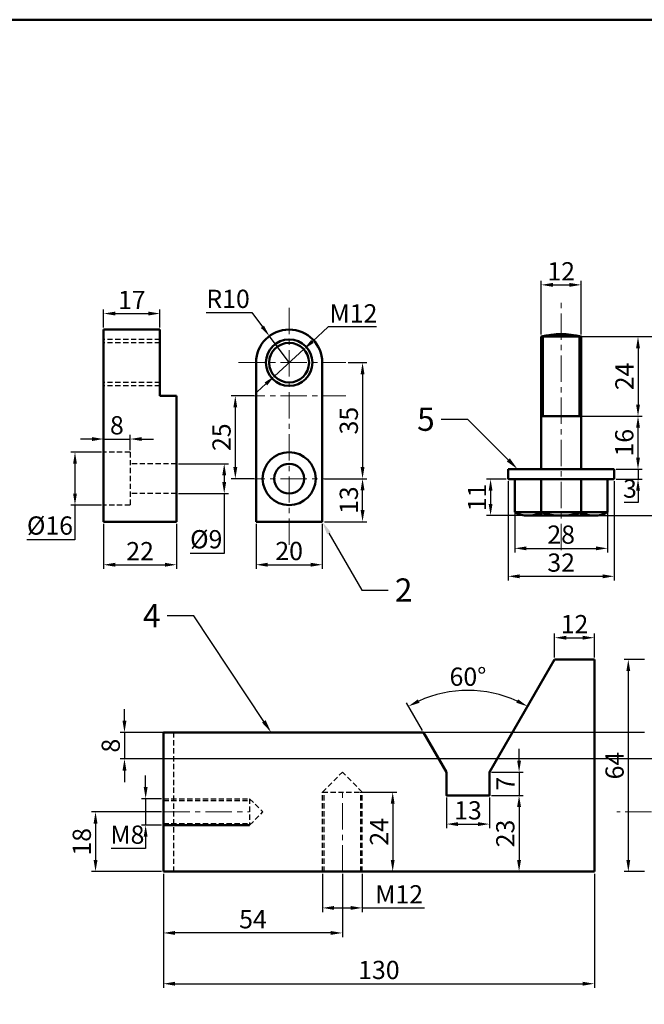
# Model space of a CAD drawing. Units: millimetres. Extents: x 10 to 613, y -226 to 271.
# Tile 3 of 4: x 251 to 439, y -26 to 271. Entities that reach past the tile are written whole.
import ezdxf
from ezdxf import colors
from ezdxf.entities.mleader import LeaderData, LeaderLine
from ezdxf.math import Vec2, Vec3

# ---------------------------------------------------------------- set-up
doc = ezdxf.new("R2010")
doc.units = ezdxf.units.MM
doc.header["$LTSCALE"] = 0.5
doc.linetypes.add('CENTER', pattern=[50.8, 31.75, -6.35, 6.35, -6.35])
doc.linetypes.add('HIDDEN', pattern=[9.525, 6.35, -3.175])
for name, color, linetype, lineweight in [('M-CNTR', 1, 'CENTER', 18), ('M-DIMS', 2, 'Continuous', 25), ('M-HIDN', 6, 'HIDDEN', 25), ('M-OUTL', 7, 'Continuous', 50), ('M-TTLB', 7, 'Continuous', 50)]:
    doc.layers.add(name, color=color, linetype=linetype, lineweight=lineweight)
doc.styles.get("Standard").update_dxf_attribs({"font": 'arial.ttf'})
doc.dimstyles.new('ISO-25', dxfattribs={"dimtxt": 5.5, "dimasz": 3.5, "dimexe": 1.25, "dimexo": 0.625, "dimtad": 1, "dimtoh": 1, "dimtxsty": 'Standard', "dimcen": 2.5, "dimadec": 0, "dimazin": 0, "dimtfac": 1, "dimtmove": 0, "dimatfit": 3, "dimfxl": 1, "dimarcsym": 0})

# ---------------------------------------------------------------- blocks, each defined once
blk = doc.blocks.new('*D5')
at = {"layer": 'Defpoints', "color": 0, "ltscale": 0.5, "transparency": 16777216}
for p in [(276.04, 140.19), (267.41, 124.19), (276.04, 124.19)]:
    blk.add_point(p, dxfattribs=at)
at = {"layer": 'M-DIMS', "color": 0, "lineweight": -2, "ltscale": 0.5, "transparency": 16777216}
for p, q in [((275.41, 140.19), (266.16, 140.19)), ((267.41, 136.69), (267.41, 127.69)), ((275.41, 124.19), (266.16, 124.19)), ((267.41, 124.19), (267.41, 113.75)), ((267.41, 113.75), (252.92, 113.75))]:
    blk.add_line(p, q, dxfattribs=at)
at = {"layer": 'M-DIMS', "color": 0, "ltscale": 0.5, "transparency": 16777216}
for points in [[(266.83, 136.69), (267.99, 136.69), (267.41, 140.19)], [(266.83, 127.69), (267.99, 127.69), (267.41, 124.19)]]:
    blk.add_solid(points, dxfattribs=at)
at = {"layer": 'M-DIMS', "color": 0, "ltscale": 0.5, "transparency": 16777216, "insert": (259.85, 117.34), "char_height": 5.5, "attachment_point": 5}
blk.add_mtext('%%C16', dxfattribs=at)
blk = doc.blocks.new('*D6')
at = {"layer": 'Defpoints', "color": 0, "ltscale": 0.5, "transparency": 16777216}
for p in [(284.04, 144.15), (276.04, 140.19), (284.04, 140.19)]:
    blk.add_point(p, dxfattribs=at)
at = {"layer": 'M-DIMS', "color": 0, "lineweight": -2, "ltscale": 0.5, "transparency": 16777216}
for p, q in [((272.54, 144.15), (269.04, 144.15)), ((276.04, 140.81), (276.04, 145.4)), ((276.04, 144.15), (284.04, 144.15)), ((284.04, 140.81), (284.04, 145.4)), ((287.54, 144.15), (291.04, 144.15))]:
    blk.add_line(p, q, dxfattribs=at)
at = {"layer": 'M-DIMS', "color": 0, "ltscale": 0.5, "transparency": 16777216}
for points in [[(272.54, 144.73), (272.54, 143.56), (276.04, 144.15)], [(287.54, 144.73), (287.54, 143.56), (284.04, 144.15)]]:
    blk.add_solid(points, dxfattribs=at)
at = {"layer": 'M-DIMS', "color": 0, "ltscale": 0.5, "transparency": 16777216, "insert": (280.04, 147.58), "char_height": 5.5, "attachment_point": 5}
blk.add_mtext('8', dxfattribs=at)
blk = doc.blocks.new('*D7')
at = {"layer": 'Defpoints', "color": 0, "ltscale": 0.5, "transparency": 16777216}
for p in [(293.04, 182), (276.04, 177.19), (293.04, 177.19)]:
    blk.add_point(p, dxfattribs=at)
at = {"layer": 'M-DIMS', "color": 0, "lineweight": -2, "ltscale": 0.5, "transparency": 16777216}
for p, q in [((276.04, 177.81), (276.04, 183.25)), ((279.54, 182), (289.54, 182)), ((293.04, 177.81), (293.04, 183.25))]:
    blk.add_line(p, q, dxfattribs=at)
at = {"layer": 'M-DIMS', "color": 0, "ltscale": 0.5, "transparency": 16777216}
for points in [[(279.54, 182.58), (279.54, 181.42), (276.04, 182)], [(289.54, 182.58), (289.54, 181.42), (293.04, 182)]]:
    blk.add_solid(points, dxfattribs=at)
at = {"layer": 'M-DIMS', "color": 0, "ltscale": 0.5, "transparency": 16777216, "insert": (284.54, 185.39), "char_height": 5.5, "attachment_point": 5}
blk.add_mtext('17', dxfattribs=at)
blk = doc.blocks.new('*D8')
at = {"layer": 'Defpoints', "color": 0, "ltscale": 0.5, "transparency": 16777216}
for p in [(298.04, 136.69), (298.04, 127.69), (312.42, 127.69)]:
    blk.add_point(p, dxfattribs=at)
at = {"layer": 'M-DIMS', "color": 0, "lineweight": -2, "ltscale": 0.5, "transparency": 16777216}
for p, q in [((298.66, 136.69), (313.67, 136.69)), ((312.42, 133.19), (312.42, 131.19)), ((298.66, 127.69), (313.67, 127.69)), ((312.42, 127.69), (312.42, 109.62)), ((312.42, 109.62), (302.2, 109.62))]:
    blk.add_line(p, q, dxfattribs=at)
at = {"layer": 'M-DIMS', "color": 0, "ltscale": 0.5, "transparency": 16777216}
for points in [[(311.84, 133.19), (313.01, 133.19), (312.42, 136.69)], [(311.84, 131.19), (313.01, 131.19), (312.42, 127.69)]]:
    blk.add_solid(points, dxfattribs=at)
at = {"layer": 'M-DIMS', "color": 0, "ltscale": 0.5, "transparency": 16777216, "insert": (307, 113.21), "char_height": 5.5, "attachment_point": 5}
blk.add_mtext('%%C9', dxfattribs=at)
blk = doc.blocks.new('*D9')
at = {"layer": 'Defpoints', "color": 0, "ltscale": 0.5, "transparency": 16777216}
for p in [(276.04, 119.19), (298.04, 119.19), (298.04, 106.22)]:
    blk.add_point(p, dxfattribs=at)
at = {"layer": 'M-DIMS', "color": 0, "lineweight": -2, "ltscale": 0.5, "transparency": 16777216}
for p, q in [((276.04, 118.56), (276.04, 104.97)), ((298.04, 118.56), (298.04, 104.97)), ((279.54, 106.22), (294.54, 106.22))]:
    blk.add_line(p, q, dxfattribs=at)
at = {"layer": 'M-DIMS', "color": 0, "ltscale": 0.5, "transparency": 16777216}
for points in [[(279.54, 106.81), (279.54, 105.64), (276.04, 106.22)], [(294.54, 106.81), (294.54, 105.64), (298.04, 106.22)]]:
    blk.add_solid(points, dxfattribs=at)
at = {"layer": 'M-DIMS', "color": 0, "ltscale": 0.5, "transparency": 16777216, "insert": (287.04, 109.61), "char_height": 5.5, "attachment_point": 5}
blk.add_mtext('22', dxfattribs=at)
blk = doc.blocks.new('*D10')
at = {"layer": 'Defpoints', "color": 0, "ltscale": 0.5, "transparency": 16777216}
for p in [(349.16, 167.19), (349.16, 132.19), (354.15, 132.19)]:
    blk.add_point(p, dxfattribs=at)
at = {"layer": 'M-DIMS', "color": 0, "lineweight": -2, "ltscale": 0.5, "transparency": 16777216}
for p, q in [((349.78, 167.19), (355.4, 167.19)), ((354.15, 163.69), (354.15, 135.69)), ((349.78, 132.19), (355.4, 132.19))]:
    blk.add_line(p, q, dxfattribs=at)
at = {"layer": 'M-DIMS', "color": 0, "ltscale": 0.5, "transparency": 16777216}
for points in [[(353.57, 163.69), (354.74, 163.69), (354.15, 167.19)], [(353.57, 135.69), (354.74, 135.69), (354.15, 132.19)]]:
    blk.add_solid(points, dxfattribs=at)
at = {"layer": 'M-DIMS', "color": 0, "ltscale": 0.5, "transparency": 16777216, "insert": (350.72, 149.69), "char_height": 5.5, "attachment_point": 5, "rotation": 90}
blk.add_mtext('35', dxfattribs=at)
blk = doc.blocks.new('*D11')
at = {"layer": 'Defpoints', "color": 0, "ltscale": 0.5, "transparency": 16777216}
for p in [(342.01, 132.19), (354.15, 132.19), (342.01, 119.19)]:
    blk.add_point(p, dxfattribs=at)
at = {"layer": 'M-DIMS', "color": 0, "lineweight": -2, "ltscale": 0.5, "transparency": 16777216}
for p, q in [((342.63, 132.19), (355.4, 132.19)), ((354.15, 122.69), (354.15, 128.69)), ((342.63, 119.19), (355.4, 119.19))]:
    blk.add_line(p, q, dxfattribs=at)
at = {"layer": 'M-DIMS', "color": 0, "ltscale": 0.5, "transparency": 16777216}
for points in [[(353.57, 128.69), (354.74, 128.69), (354.15, 132.19)], [(353.57, 122.69), (354.74, 122.69), (354.15, 119.19)]]:
    blk.add_solid(points, dxfattribs=at)
at = {"layer": 'M-DIMS', "color": 0, "ltscale": 0.5, "transparency": 16777216, "insert": (350.72, 125.69), "char_height": 5.5, "attachment_point": 5, "rotation": 90}
blk.add_mtext('13', dxfattribs=at)
blk = doc.blocks.new('*D12')
at = {"layer": 'Defpoints', "color": 0, "ltscale": 0.5, "transparency": 16777216}
for p in [(322.01, 119.19), (342.01, 119.19), (342.01, 106.22)]:
    blk.add_point(p, dxfattribs=at)
at = {"layer": 'M-DIMS', "color": 0, "lineweight": -2, "ltscale": 0.5, "transparency": 16777216}
for p, q in [((322.01, 118.56), (322.01, 104.97)), ((342.01, 118.56), (342.01, 104.97)), ((325.51, 106.22), (338.51, 106.22))]:
    blk.add_line(p, q, dxfattribs=at)
at = {"layer": 'M-DIMS', "color": 0, "ltscale": 0.5, "transparency": 16777216}
for points in [[(325.51, 106.81), (325.51, 105.64), (322.01, 106.22)], [(338.51, 106.81), (338.51, 105.64), (342.01, 106.22)]]:
    blk.add_solid(points, dxfattribs=at)
at = {"layer": 'M-DIMS', "color": 0, "ltscale": 0.5, "transparency": 16777216, "insert": (332.01, 109.66), "char_height": 5.5, "attachment_point": 5}
blk.add_mtext('20', dxfattribs=at)
blk = doc.blocks.new('*D13')
at = {"layer": 'Defpoints', "color": 0, "ltscale": 0.5, "transparency": 16777216}
for p in [(322.01, 157.19), (315.77, 132.19), (322.01, 132.19)]:
    blk.add_point(p, dxfattribs=at)
at = {"layer": 'M-DIMS', "color": 0, "lineweight": -2, "ltscale": 0.5, "transparency": 16777216}
for p, q in [((321.38, 157.19), (314.52, 157.19)), ((315.77, 153.69), (315.77, 135.69)), ((321.38, 132.19), (314.52, 132.19))]:
    blk.add_line(p, q, dxfattribs=at)
at = {"layer": 'M-DIMS', "color": 0, "ltscale": 0.5, "transparency": 16777216}
for points in [[(315.18, 153.69), (316.35, 153.69), (315.77, 157.19)], [(315.18, 135.69), (316.35, 135.69), (315.77, 132.19)]]:
    blk.add_solid(points, dxfattribs=at)
at = {"layer": 'M-DIMS', "color": 0, "ltscale": 0.5, "transparency": 16777216, "insert": (312.33, 144.69), "char_height": 5.5, "attachment_point": 5, "rotation": 90}
blk.add_mtext('25', dxfattribs=at)
blk = doc.blocks.new('*D14')
at = {"layer": 'Defpoints', "color": 0, "ltscale": 0.5, "transparency": 16777216}
for p in [(326.04, 175.21), (332.01, 167.19)]:
    blk.add_point(p, dxfattribs=at)
at = {"layer": 'M-DIMS', "color": 0, "lineweight": -2, "ltscale": 0.5, "transparency": 16777216}
for p, q in [((307.02, 182.3), (320.77, 182.3)), ((320.77, 182.3), (323.95, 178.02)), ((332.01, 167.19), (326.04, 175.21))]:
    blk.add_line(p, q, dxfattribs=at)
at = {"layer": 'M-DIMS', "color": 0, "ltscale": 0.5, "transparency": 16777216}
blk.add_solid([(324.42, 178.37), (323.48, 177.67), (326.04, 175.21)], dxfattribs=at)
at = {"layer": 'M-DIMS', "color": 0, "ltscale": 0.5, "transparency": 16777216, "insert": (313.58, 185.73), "char_height": 5.5, "attachment_point": 5}
blk.add_mtext('R10', dxfattribs=at)
blk = doc.blocks.new('*D15')
at = {"layer": 'Defpoints', "color": 0, "ltscale": 0.5, "transparency": 16777216}
for p in [(336.44, 171.23), (327.58, 163.14)]:
    blk.add_point(p, dxfattribs=at)
at = {"layer": 'M-DIMS', "color": 0, "lineweight": -2, "ltscale": 0.5, "transparency": 16777216}
for p, q in [((343.8, 177.96), (339.02, 173.6)), ((358.4, 177.96), (343.8, 177.96)), ((327.58, 163.14), (336.44, 171.23)), ((324.99, 160.78), (322.41, 158.42))]:
    blk.add_line(p, q, dxfattribs=at)
at = {"layer": 'M-DIMS', "color": 0, "ltscale": 0.5, "transparency": 16777216}
for points in [[(338.63, 174.03), (339.42, 173.16), (336.44, 171.23)], [(324.6, 161.21), (325.39, 160.35), (327.58, 163.14)]]:
    blk.add_solid(points, dxfattribs=at)
at = {"layer": 'M-DIMS', "color": 0, "ltscale": 0.5, "transparency": 16777216, "insert": (351.41, 181.34), "char_height": 5.5, "attachment_point": 5}
blk.add_mtext('M12', dxfattribs=at)
blk = doc.blocks.new('*D24')
at = {"layer": 'Defpoints', "color": 0, "ltscale": 0.5, "transparency": 16777216}
for p in [(294.08, 13.64), (424.08, 13.64), (424.08, -20.18)]:
    blk.add_point(p, dxfattribs=at)
at = {"layer": 'M-DIMS', "color": 0, "lineweight": -2, "ltscale": 0.5, "transparency": 16777216}
for p, q in [((294.08, 13.02), (294.08, -21.43)), ((424.08, 13.02), (424.08, -21.43)), ((297.58, -20.18), (420.58, -20.18))]:
    blk.add_line(p, q, dxfattribs=at)
at = {"layer": 'M-DIMS', "color": 0, "ltscale": 0.5, "transparency": 16777216}
for points in [[(297.58, -19.6), (297.58, -20.76), (294.08, -20.18)], [(420.58, -19.6), (420.58, -20.76), (424.08, -20.18)]]:
    blk.add_solid(points, dxfattribs=at)
at = {"layer": 'M-DIMS', "color": 0, "ltscale": 0.5, "transparency": 16777216, "insert": (359.08, -16.74), "char_height": 5.5, "attachment_point": 5}
blk.add_mtext('130', dxfattribs=at)
blk = doc.blocks.new('*D25')
at = {"layer": 'Defpoints', "color": 0, "ltscale": 0.5, "transparency": 16777216}
for p in [(294.08, 13.64), (348.08, 13.64), (294.08, -4.86)]:
    blk.add_point(p, dxfattribs=at)
at = {"layer": 'M-DIMS', "color": 0, "lineweight": -2, "ltscale": 0.5, "transparency": 16777216}
for p, q in [((294.08, 13.02), (294.08, -6.11)), ((348.08, 13.02), (348.08, -6.11)), ((344.58, -4.86), (297.58, -4.86))]:
    blk.add_line(p, q, dxfattribs=at)
at = {"layer": 'M-DIMS', "color": 0, "ltscale": 0.5, "transparency": 16777216}
for points in [[(297.58, -4.28), (297.58, -5.44), (294.08, -4.86)], [(344.58, -4.28), (344.58, -5.44), (348.08, -4.86)]]:
    blk.add_solid(points, dxfattribs=at)
at = {"layer": 'M-DIMS', "color": 0, "ltscale": 0.5, "transparency": 16777216, "insert": (321.08, -1.44), "char_height": 5.5, "attachment_point": 5}
blk.add_mtext('54', dxfattribs=at)
blk = doc.blocks.new('*D26')
at = {"layer": 'Defpoints', "color": 0, "ltscale": 0.5, "transparency": 16777216}
for p in [(342.08, 13.64), (354.08, 13.64), (354.08, 2.69)]:
    blk.add_point(p, dxfattribs=at)
at = {"layer": 'M-DIMS', "color": 0, "lineweight": -2, "ltscale": 0.5, "transparency": 16777216}
for p, q in [((342.08, 13.02), (342.08, 1.44)), ((354.08, 13.02), (354.08, 1.44)), ((345.58, 2.69), (350.58, 2.69)), ((354.08, 2.69), (372.81, 2.69))]:
    blk.add_line(p, q, dxfattribs=at)
at = {"layer": 'M-DIMS', "color": 0, "ltscale": 0.5, "transparency": 16777216}
for points in [[(345.58, 3.27), (345.58, 2.11), (342.08, 2.69)], [(350.58, 3.27), (350.58, 2.11), (354.08, 2.69)]]:
    blk.add_solid(points, dxfattribs=at)
at = {"layer": 'M-DIMS', "color": 0, "ltscale": 0.5, "transparency": 16777216, "insert": (365.19, 6.08), "char_height": 5.5, "attachment_point": 5}
blk.add_mtext('M12', dxfattribs=at)
blk = doc.blocks.new('*D27')
at = {"layer": 'Defpoints', "color": 0, "ltscale": 0.5, "transparency": 16777216}
for p in [(353.58, 37.64), (353.58, 13.64), (363.24, 13.64)]:
    blk.add_point(p, dxfattribs=at)
at = {"layer": 'M-DIMS', "color": 0, "lineweight": -2, "ltscale": 0.5, "transparency": 16777216}
for p, q in [((354.21, 37.64), (364.49, 37.64)), ((363.24, 34.14), (363.24, 17.14)), ((354.21, 13.64), (364.49, 13.64))]:
    blk.add_line(p, q, dxfattribs=at)
at = {"layer": 'M-DIMS', "color": 0, "ltscale": 0.5, "transparency": 16777216}
for points in [[(362.66, 34.14), (363.82, 34.14), (363.24, 37.64)], [(362.66, 17.14), (363.82, 17.14), (363.24, 13.64)]]:
    blk.add_solid(points, dxfattribs=at)
at = {"layer": 'M-DIMS', "color": 0, "ltscale": 0.5, "transparency": 16777216, "insert": (359.85, 25.64), "char_height": 5.5, "attachment_point": 5, "rotation": 90}
blk.add_mtext('24', dxfattribs=at)
blk = doc.blocks.new('*D28')
at = {"layer": 'Defpoints', "color": 0, "ltscale": 0.5, "transparency": 16777216}
for p in [(294.08, 35.64), (288.72, 27.64), (294.08, 27.64)]:
    blk.add_point(p, dxfattribs=at)
at = {"layer": 'M-DIMS', "color": 0, "lineweight": -2, "ltscale": 0.5, "transparency": 16777216}
for p, q in [((288.72, 39.14), (288.72, 42.64)), ((293.46, 35.64), (287.47, 35.64)), ((288.72, 35.64), (288.72, 27.64)), ((293.46, 27.64), (287.47, 27.64)), ((288.72, 24.14), (288.72, 20.64)), ((288.72, 20.64), (278.33, 20.64))]:
    blk.add_line(p, q, dxfattribs=at)
at = {"layer": 'M-DIMS', "color": 0, "ltscale": 0.5, "transparency": 16777216}
for points in [[(288.14, 39.14), (289.3, 39.14), (288.72, 35.64)], [(288.14, 24.14), (289.3, 24.14), (288.72, 27.64)]]:
    blk.add_solid(points, dxfattribs=at)
at = {"layer": 'M-DIMS', "color": 0, "ltscale": 0.5, "transparency": 16777216, "insert": (283.21, 24.08), "char_height": 5.5, "attachment_point": 5}
blk.add_mtext('M8', dxfattribs=at)
blk = doc.blocks.new('*D29')
at = {"layer": 'Defpoints', "color": 0, "ltscale": 0.5, "transparency": 16777216}
for p in [(294.08, 31.64), (273.6, 13.64), (294.08, 13.64)]:
    blk.add_point(p, dxfattribs=at)
at = {"layer": 'M-DIMS', "color": 0, "lineweight": -2, "ltscale": 0.5, "transparency": 16777216}
for p, q in [((293.46, 31.64), (272.35, 31.64)), ((273.6, 28.14), (273.6, 17.14)), ((293.46, 13.64), (272.35, 13.64))]:
    blk.add_line(p, q, dxfattribs=at)
at = {"layer": 'M-DIMS', "color": 0, "ltscale": 0.5, "transparency": 16777216}
for points in [[(273.02, 28.14), (274.19, 28.14), (273.6, 31.64)], [(273.02, 17.14), (274.19, 17.14), (273.6, 13.64)]]:
    blk.add_solid(points, dxfattribs=at)
at = {"layer": 'M-DIMS', "color": 0, "ltscale": 0.5, "transparency": 16777216, "insert": (270.17, 22.64), "char_height": 5.5, "attachment_point": 5, "rotation": 90}
blk.add_mtext('18', dxfattribs=at)
blk = doc.blocks.new('*D30')
at = {"layer": 'Defpoints', "color": 0, "ltscale": 0.5, "transparency": 16777216}
for p in [(392.45, 36.64), (392.45, 13.64), (401.37, 13.64)]:
    blk.add_point(p, dxfattribs=at)
at = {"layer": 'M-DIMS', "color": 0, "lineweight": -2, "ltscale": 0.5, "transparency": 16777216}
for p, q in [((393.08, 36.64), (402.62, 36.64)), ((401.37, 33.14), (401.37, 17.14)), ((393.08, 13.64), (402.62, 13.64))]:
    blk.add_line(p, q, dxfattribs=at)
at = {"layer": 'M-DIMS', "color": 0, "ltscale": 0.5, "transparency": 16777216}
for points in [[(400.78, 33.14), (401.95, 33.14), (401.37, 36.64)], [(400.78, 17.14), (401.95, 17.14), (401.37, 13.64)]]:
    blk.add_solid(points, dxfattribs=at)
at = {"layer": 'M-DIMS', "color": 0, "ltscale": 0.5, "transparency": 16777216, "insert": (397.93, 25.14), "char_height": 5.5, "attachment_point": 5, "rotation": 90}
blk.add_mtext('23', dxfattribs=at)
blk = doc.blocks.new('*D31')
at = {"layer": 'Defpoints', "color": 0, "ltscale": 0.5, "transparency": 16777216}
for p in [(379.45, 36.64), (392.45, 36.64), (392.45, 27.98)]:
    blk.add_point(p, dxfattribs=at)
at = {"layer": 'M-DIMS', "color": 0, "lineweight": -2, "ltscale": 0.5, "transparency": 16777216}
for p, q in [((379.45, 36.02), (379.45, 26.73)), ((392.45, 36.02), (392.45, 26.73)), ((382.95, 27.98), (388.95, 27.98))]:
    blk.add_line(p, q, dxfattribs=at)
at = {"layer": 'M-DIMS', "color": 0, "ltscale": 0.5, "transparency": 16777216}
for points in [[(382.95, 28.56), (382.95, 27.39), (379.45, 27.98)], [(388.95, 28.56), (388.95, 27.39), (392.45, 27.98)]]:
    blk.add_solid(points, dxfattribs=at)
at = {"layer": 'M-DIMS', "color": 0, "ltscale": 0.5, "transparency": 16777216, "insert": (385.95, 31.41), "char_height": 5.5, "attachment_point": 5}
blk.add_mtext('13', dxfattribs=at)
blk = doc.blocks.new('*D32')
at = {"layer": 'Defpoints', "color": 0, "ltscale": 0.5, "transparency": 16777216}
for p in [(392.45, 43.64), (392.45, 36.64), (401.37, 36.64)]:
    blk.add_point(p, dxfattribs=at)
at = {"layer": 'M-DIMS', "color": 0, "lineweight": -2, "ltscale": 0.5, "transparency": 16777216}
for p, q in [((401.37, 47.14), (401.37, 50.64)), ((393.08, 43.64), (402.62, 43.64)), ((401.37, 43.64), (401.37, 36.64)), ((393.08, 36.64), (402.62, 36.64)), ((401.37, 33.14), (401.37, 29.64))]:
    blk.add_line(p, q, dxfattribs=at)
at = {"layer": 'M-DIMS', "color": 0, "ltscale": 0.5, "transparency": 16777216}
for points in [[(400.78, 47.14), (401.95, 47.14), (401.37, 43.64)], [(400.78, 33.14), (401.95, 33.14), (401.37, 36.64)]]:
    blk.add_solid(points, dxfattribs=at)
at = {"layer": 'M-DIMS', "color": 0, "ltscale": 0.5, "transparency": 16777216, "insert": (397.99, 40.14), "char_height": 5.5, "attachment_point": 5, "rotation": 90}
blk.add_mtext('7', dxfattribs=at)
blk = doc.blocks.new('*D33')
at = {"layer": 'Defpoints', "color": 0, "ltscale": 0.5, "transparency": 16777216}
for p in [(424.08, 84.21), (412.08, 77.64), (424.08, 77.64)]:
    blk.add_point(p, dxfattribs=at)
at = {"layer": 'M-DIMS', "color": 0, "lineweight": -2, "ltscale": 0.5, "transparency": 16777216}
for p, q in [((412.08, 78.27), (412.08, 85.46)), ((415.58, 84.21), (420.58, 84.21)), ((424.08, 78.27), (424.08, 85.46))]:
    blk.add_line(p, q, dxfattribs=at)
at = {"layer": 'M-DIMS', "color": 0, "ltscale": 0.5, "transparency": 16777216}
for points in [[(415.58, 84.79), (415.58, 83.62), (412.08, 84.21)], [(420.58, 84.79), (420.58, 83.62), (424.08, 84.21)]]:
    blk.add_solid(points, dxfattribs=at)
at = {"layer": 'M-DIMS', "color": 0, "ltscale": 0.5, "transparency": 16777216, "insert": (418.08, 87.59), "char_height": 5.5, "attachment_point": 5}
blk.add_mtext('12', dxfattribs=at)
blk = doc.blocks.new('*D34')
at = {"layer": 'Defpoints', "color": 0, "ltscale": 0.5, "transparency": 16777216}
for p in [(412.08, 77.64), (392.19, 67.76), (372.53, 55.64), (379.45, 43.64), (392.45, 43.64)]:
    blk.add_point(p, dxfattribs=at)
at = {"layer": 'M-DIMS', "color": 0, "lineweight": -2, "ltscale": 0.5, "transparency": 16777216}
blk.add_line((372.21, 56.18), (367.37, 64.58), dxfattribs=at)
blk.add_arc((385.95, 32.38), 35.93, 65.5841, 114.4159, dxfattribs=at)
at = {"layer": 'M-DIMS', "color": 0, "ltscale": 0.5, "transparency": 16777216}
for points in [[(371.37, 64.58), (370.84, 65.62), (367.99, 63.5)], [(401.07, 65.62), (400.54, 64.58), (403.92, 63.5)]]:
    blk.add_solid(points, dxfattribs=at)
at = {"layer": 'M-DIMS', "color": 0, "ltscale": 0.5, "transparency": 16777216, "insert": (385.95, 71.74), "char_height": 5.5, "attachment_point": 5}
blk.add_mtext('60°', dxfattribs=at)
blk = doc.blocks.new('*D35')
at = {"layer": 'Defpoints', "color": 0, "ltscale": 0.5, "transparency": 16777216}
for p in [(439.79, 77.64), (434.32, 13.64), (439.79, 13.64)]:
    blk.add_point(p, dxfattribs=at)
at = {"layer": 'M-DIMS', "color": 0, "lineweight": -2, "ltscale": 0.5, "transparency": 16777216}
for p, q in [((439.17, 77.64), (433.07, 77.64)), ((434.32, 74.14), (434.32, 17.14)), ((439.17, 13.64), (433.07, 13.64))]:
    blk.add_line(p, q, dxfattribs=at)
at = {"layer": 'M-DIMS', "color": 0, "ltscale": 0.5, "transparency": 16777216}
for points in [[(433.74, 74.14), (434.9, 74.14), (434.32, 77.64)], [(433.74, 17.14), (434.9, 17.14), (434.32, 13.64)]]:
    blk.add_solid(points, dxfattribs=at)
at = {"layer": 'M-DIMS', "color": 0, "ltscale": 0.5, "transparency": 16777216, "insert": (430.89, 45.64), "char_height": 5.5, "attachment_point": 5, "rotation": 90}
blk.add_mtext('64', dxfattribs=at)
blk = doc.blocks.new('*D39')
at = {"layer": 'Defpoints', "color": 0, "ltscale": 0.5, "transparency": 16777216}
for p in [(400.06, 127.04), (428.06, 127.04), (428.06, 111.17)]:
    blk.add_point(p, dxfattribs=at)
at = {"layer": 'M-DIMS', "color": 0, "lineweight": -2, "ltscale": 0.5, "transparency": 16777216}
for p, q in [((400.06, 126.42), (400.06, 109.92)), ((428.06, 126.42), (428.06, 109.92)), ((403.56, 111.17), (424.56, 111.17))]:
    blk.add_line(p, q, dxfattribs=at)
at = {"layer": 'M-DIMS', "color": 0, "ltscale": 0.5, "transparency": 16777216}
for points in [[(403.56, 111.75), (403.56, 110.59), (400.06, 111.17)], [(424.56, 111.75), (424.56, 110.59), (428.06, 111.17)]]:
    blk.add_solid(points, dxfattribs=at)
at = {"layer": 'M-DIMS', "color": 0, "ltscale": 0.5, "transparency": 16777216, "insert": (414.06, 114.6), "char_height": 5.5, "attachment_point": 5}
blk.add_mtext('28', dxfattribs=at)
blk = doc.blocks.new('*D40')
at = {"layer": 'Defpoints', "color": 0, "ltscale": 0.5, "transparency": 16777216}
for p in [(398.06, 132.04), (430.06, 132.04), (430.06, 102.73)]:
    blk.add_point(p, dxfattribs=at)
at = {"layer": 'M-DIMS', "color": 0, "lineweight": -2, "ltscale": 0.5, "transparency": 16777216}
for p, q in [((398.06, 131.42), (398.06, 101.48)), ((430.06, 131.42), (430.06, 101.48)), ((401.56, 102.73), (426.56, 102.73))]:
    blk.add_line(p, q, dxfattribs=at)
at = {"layer": 'M-DIMS', "color": 0, "ltscale": 0.5, "transparency": 16777216}
for points in [[(401.56, 103.31), (401.56, 102.14), (398.06, 102.73)], [(426.56, 103.31), (426.56, 102.14), (430.06, 102.73)]]:
    blk.add_solid(points, dxfattribs=at)
at = {"layer": 'M-DIMS', "color": 0, "ltscale": 0.5, "transparency": 16777216, "insert": (414.06, 106.16), "char_height": 5.5, "attachment_point": 5}
blk.add_mtext('32', dxfattribs=at)
blk = doc.blocks.new('*D41')
at = {"layer": 'Defpoints', "color": 0, "ltscale": 0.5, "transparency": 16777216}
for p in [(420.06, 151.04), (437.24, 151.04), (430.06, 135.04)]:
    blk.add_point(p, dxfattribs=at)
at = {"layer": 'M-DIMS', "color": 0, "lineweight": -2, "ltscale": 0.5, "transparency": 16777216}
for p, q in [((420.68, 151.04), (438.49, 151.04)), ((437.24, 138.54), (437.24, 147.54)), ((430.68, 135.04), (438.49, 135.04))]:
    blk.add_line(p, q, dxfattribs=at)
at = {"layer": 'M-DIMS', "color": 0, "ltscale": 0.5, "transparency": 16777216}
for points in [[(436.66, 147.54), (437.83, 147.54), (437.24, 151.04)], [(436.66, 138.54), (437.83, 138.54), (437.24, 135.04)]]:
    blk.add_solid(points, dxfattribs=at)
at = {"layer": 'M-DIMS', "color": 0, "ltscale": 0.5, "transparency": 16777216, "insert": (433.81, 143.04), "char_height": 5.5, "attachment_point": 5, "rotation": 90}
blk.add_mtext('16', dxfattribs=at)
blk = doc.blocks.new('*D42')
at = {"layer": 'Defpoints', "color": 0, "ltscale": 0.5, "transparency": 16777216}
for p in [(430.06, 135.04), (430.06, 132.04), (437.24, 132.04)]:
    blk.add_point(p, dxfattribs=at)
at = {"layer": 'M-DIMS', "color": 0, "lineweight": -2, "ltscale": 0.5, "transparency": 16777216}
for p, q in [((437.24, 138.54), (437.24, 142.04)), ((430.68, 135.04), (438.49, 135.04)), ((437.24, 135.04), (437.24, 132.04)), ((430.68, 132.04), (438.49, 132.04)), ((437.24, 128.54), (437.24, 125.04)), ((437.24, 125.04), (433.02, 125.04))]:
    blk.add_line(p, q, dxfattribs=at)
at = {"layer": 'M-DIMS', "color": 0, "ltscale": 0.5, "transparency": 16777216}
for points in [[(436.66, 138.54), (437.83, 138.54), (437.24, 135.04)], [(436.66, 128.54), (437.83, 128.54), (437.24, 132.04)]]:
    blk.add_solid(points, dxfattribs=at)
at = {"layer": 'M-DIMS', "color": 0, "ltscale": 0.5, "transparency": 16777216, "insert": (434.82, 128.48), "char_height": 5.5, "attachment_point": 5}
blk.add_mtext('3', dxfattribs=at)
blk = doc.blocks.new('*D43')
at = {"layer": 'Defpoints', "color": 0, "ltscale": 0.5, "transparency": 16777216}
for p in [(398.06, 132.04), (392.77, 121.04), (408.06, 121.04)]:
    blk.add_point(p, dxfattribs=at)
at = {"layer": 'M-DIMS', "color": 0, "lineweight": -2, "ltscale": 0.5, "transparency": 16777216}
for p, q in [((397.43, 132.04), (391.52, 132.04)), ((392.77, 128.54), (392.77, 124.54)), ((407.43, 121.04), (391.52, 121.04))]:
    blk.add_line(p, q, dxfattribs=at)
at = {"layer": 'M-DIMS', "color": 0, "ltscale": 0.5, "transparency": 16777216}
for points in [[(392.19, 128.54), (393.35, 128.54), (392.77, 132.04)], [(392.19, 124.54), (393.35, 124.54), (392.77, 121.04)]]:
    blk.add_solid(points, dxfattribs=at)
at = {"layer": 'M-DIMS', "color": 0, "ltscale": 0.5, "transparency": 16777216, "insert": (389.38, 126.54), "char_height": 5.5, "attachment_point": 5, "rotation": 90}
blk.add_mtext('11', dxfattribs=at)
blk = doc.blocks.new('*D44')
at = {"layer": 'Defpoints', "color": 0, "ltscale": 0.5, "transparency": 16777216}
for p in [(420.06, 175.04), (419.56, 151.04), (437.24, 151.04)]:
    blk.add_point(p, dxfattribs=at)
at = {"layer": 'M-DIMS', "color": 0, "lineweight": -2, "ltscale": 0.5, "transparency": 16777216}
for p, q in [((420.68, 175.04), (438.49, 175.04)), ((437.24, 171.54), (437.24, 154.54)), ((420.18, 151.04), (438.49, 151.04))]:
    blk.add_line(p, q, dxfattribs=at)
at = {"layer": 'M-DIMS', "color": 0, "ltscale": 0.5, "transparency": 16777216}
for points in [[(436.66, 171.54), (437.83, 171.54), (437.24, 175.04)], [(436.66, 154.54), (437.83, 154.54), (437.24, 151.04)]]:
    blk.add_solid(points, dxfattribs=at)
at = {"layer": 'M-DIMS', "color": 0, "ltscale": 0.5, "transparency": 16777216, "insert": (433.86, 163.04), "char_height": 5.5, "attachment_point": 5, "rotation": 90}
blk.add_mtext('24', dxfattribs=at)
blk = doc.blocks.new('*D45')
at = {"layer": 'Defpoints', "color": 0, "ltscale": 0.5, "transparency": 16777216}
for p in [(414.06, 175.04), (414.06, 121.04), (449.51, 121.04)]:
    blk.add_point(p, dxfattribs=at)
at = {"layer": 'M-DIMS', "color": 0, "lineweight": -2, "ltscale": 0.5, "transparency": 16777216}
for p, q in [((414.68, 175.04), (450.76, 175.04)), ((449.51, 171.54), (449.51, 124.54)), ((414.68, 121.04), (450.76, 121.04))]:
    blk.add_line(p, q, dxfattribs=at)
at = {"layer": 'M-DIMS', "color": 0, "ltscale": 0.5, "transparency": 16777216}
for points in [[(448.93, 171.54), (450.09, 171.54), (449.51, 175.04)], [(448.93, 124.54), (450.09, 124.54), (449.51, 121.04)]]:
    blk.add_solid(points, dxfattribs=at)
at = {"layer": 'M-DIMS', "color": 0, "ltscale": 0.5, "transparency": 16777216, "insert": (446.09, 148.04), "char_height": 5.5, "attachment_point": 5, "rotation": 90}
blk.add_mtext('54', dxfattribs=at)
blk = doc.blocks.new('*D58')
at = {"layer": 'Defpoints', "color": 0, "ltscale": 0.5, "transparency": 16777216}
for p in [(420.06, 190.66), (408.06, 175.04), (420.06, 175.04)]:
    blk.add_point(p, dxfattribs=at)
at = {"layer": 'M-DIMS', "color": 0, "lineweight": -2, "ltscale": 0.5, "transparency": 16777216}
for p, q in [((408.06, 175.67), (408.06, 191.91)), ((411.56, 190.66), (416.56, 190.66)), ((420.06, 175.67), (420.06, 191.91))]:
    blk.add_line(p, q, dxfattribs=at)
at = {"layer": 'M-DIMS', "color": 0, "ltscale": 0.5, "transparency": 16777216}
for points in [[(411.56, 191.24), (411.56, 190.07), (408.06, 190.66)], [(416.56, 191.24), (416.56, 190.07), (420.06, 190.66)]]:
    blk.add_solid(points, dxfattribs=at)
at = {"layer": 'M-DIMS', "color": 0, "ltscale": 0.5, "transparency": 16777216, "insert": (414.06, 194.04), "char_height": 5.5, "attachment_point": 5}
blk.add_mtext('12', dxfattribs=at)
blk = doc.blocks.new('*D61')
at = {"layer": 'Defpoints', "color": 0, "ltscale": 0.5, "transparency": 16777216}
for p in [(439.79, 55.64), (282.33, 47.64), (449.79, 47.64)]:
    blk.add_point(p, dxfattribs=at)
at = {"layer": 'M-DIMS', "color": 0, "lineweight": -2, "ltscale": 0.5, "transparency": 16777216}
for p, q in [((282.33, 59.14), (282.33, 62.64)), ((439.17, 55.64), (281.08, 55.64)), ((282.33, 55.64), (282.33, 47.64)), ((449.17, 47.64), (281.08, 47.64)), ((282.33, 44.14), (282.33, 40.64))]:
    blk.add_line(p, q, dxfattribs=at)
at = {"layer": 'M-DIMS', "color": 0, "ltscale": 0.5, "transparency": 16777216}
for points in [[(281.75, 59.14), (282.92, 59.14), (282.33, 55.64)], [(281.75, 44.14), (282.92, 44.14), (282.33, 47.64)]]:
    blk.add_solid(points, dxfattribs=at)
at = {"layer": 'M-DIMS', "color": 0, "ltscale": 0.5, "transparency": 16777216, "insert": (278.9, 51.64), "char_height": 5.5, "attachment_point": 5, "rotation": 90}
blk.add_mtext('8', dxfattribs=at)

msp = doc.modelspace()

# ---------------------------------------------------------------- linework, layer by layer
at = {"layer": 'M-CNTR', "ltscale": 0.5}
for p, q in [((414.058, 110.611), (414.058, 186.255)), ((332.009, 183.694), (332.009, 111.752)), ((316.736, 167.189), (349.155, 167.189)), ((316.736, 157.189), (349.155, 157.189)), ((316.736, 132.189), (349.155, 132.189)), ((348.084, 13.642), (348.084, 37.642)), ((294.084, 31.642), (320.084, 31.642)), ((504.837, 31.642), (430.858, 31.642))]:
    msp.add_line(p, q, dxfattribs=at)
at = {"layer": 'M-HIDN', "ltscale": 0.5}
for p, q in [((293.039, 174.189), (276.039, 174.189)), ((293.039, 173.189), (276.039, 173.189)), ((293.039, 161.189), (276.039, 161.189)), ((293.039, 160.189), (276.039, 160.189)), ((284.039, 140.189), (276.039, 140.189)), ((284.039, 140.189), (284.039, 124.189)), ((298.039, 136.689), (284.039, 136.689)), ((298.039, 127.689), (284.039, 127.689)), ((284.039, 124.189), (276.039, 124.189)), ((297.084, 55.642), (297.084, 13.642)), ((377.145, 47.642), (294.084, 47.642)), ((342.084, 37.642), (348.084, 43.642)), ((354.084, 37.642), (348.084, 43.642)), ((342.084, 13.642), (342.084, 37.642)), ((342.084, 37.642), (354.084, 37.642)), ((342.584, 13.642), (342.584, 37.642)), ((353.584, 13.642), (353.584, 37.642)), ((354.084, 13.642), (354.084, 37.642)), ((294.084, 35.642), (320.084, 35.642)), ((294.084, 35.142), (320.084, 35.142)), ((320.084, 35.642), (320.084, 27.642)), ((320.084, 35.642), (324.084, 31.642)), ((320.084, 27.642), (324.084, 31.642)), ((294.084, 28.142), (320.084, 28.142))]:
    msp.add_line(p, q, dxfattribs=at)
at = {"layer": 'M-OUTL', "ltscale": 0.5}
for p, q in [((293.039, 177.189), (276.039, 177.189)), ((276.039, 177.189), (276.039, 119.189)), ((293.039, 157.189), (293.039, 177.189)), ((414.058, 175.041), (408.058, 175.041)), ((408.058, 175.041), (408.058, 135.041)), ((408.558, 175.041), (408.558, 151.041)), ((414.058, 175.041), (420.058, 175.041)), ((419.558, 175.041), (419.558, 151.041)), ((420.058, 175.041), (420.058, 135.041)), ((322.009, 167.189), (322.009, 119.189)), ((342.009, 167.189), (342.009, 119.189)), ((298.039, 157.189), (293.039, 157.189)), ((298.039, 119.189), (298.039, 157.189)), ((408.058, 151.041), (420.058, 151.041)), ((398.058, 135.041), (430.058, 135.041)), ((398.058, 132.041), (398.058, 135.041)), ((430.058, 135.041), (430.058, 132.041)), ((430.058, 132.041), (398.058, 132.041)), ((400.058, 132.041), (428.058, 132.041)), ((400.058, 122.041), (400.058, 132.041)), ((408.058, 132.041), (408.058, 121.041)), ((420.058, 132.041), (420.058, 121.041)), ((428.058, 132.041), (428.058, 122.041)), ((428.058, 122.041), (400.058, 122.041)), ((276.039, 119.189), (298.039, 119.189)), ((322.009, 119.189), (342.009, 119.189)), ((424.182, 121.041), (403.934, 121.041)), ((424.084, 77.642), (412.084, 77.642)), ((424.084, 13.642), (424.084, 77.642)), ((294.084, 13.642), (294.084, 55.642)), ((294.084, 55.642), (372.526, 55.642)), ((294.084, 27.642), (320.084, 27.642)), ((424.084, 13.642), (294.084, 13.642)), ((398.889, 13.642), (424.084, 13.642))]:
    msp.add_line(p, q, dxfattribs=at)
msp.add_lwpolyline([(372.526, 55.642), (379.454, 43.642), (379.454, 36.642), (392.454, 36.642), (392.454, 43.642), (412.084, 77.642)], dxfattribs=at)
for centre, radius in [((332.009, 167.189), 7), ((332.009, 167.189), 6), ((332.009, 132.189), 8), ((332.009, 132.189), 4.5)]:
    msp.add_circle(centre, radius, dxfattribs=at)
for centre, radius, start, end in [((332.009, 167.189), 10, 0, 180), ((414.058, 151.474), 24.318, 75.71605, 104.28395), ((404.058, 129.533), 8.493, 241.90309, 298.09691), ((414.058, 139.541), 18.5, 251.07536, 288.92464), ((424.058, 129.533), 8.493, 241.90309, 298.09691)]:
    msp.add_arc(centre, radius, start, end, dxfattribs=at)
at = {"layer": 'M-TTLB', "ltscale": 0.5}
msp.add_lwpolyline([(9.692, 270.659), (613.416, 270.659), (613.416, -225.522), (9.692, -225.522)], close=True, dxfattribs=at)

# ---------------------------------------------------------------- dimensions: what is measured, and where the dimension line sits
at = {"layer": 'M-DIMS', "ltscale": 0.5}
for base, p1, p2, override, picture, middle in [((420.058, 190.655), (408.058, 175.041), (420.058, 175.041), {"dimdec": 0, "dimlfac": 1, "dimrnd": 0, "dimzin": 0, "dimdsep": 46, "dimlunit": 2}, '*D58', (414.058, 194.042)), ((293.039, 182), (276.039, 177.189), (293.039, 177.189), {"dimclrd": 0, "dimclre": 0, "dimclrt": 0}, '*D7', (284.539, 185.386)), ((284.039, 144.145), (276.039, 140.189), (284.039, 140.189), {"dimclrd": 0, "dimclre": 0, "dimclrt": 0}, '*D6', (280.039, 147.578)), ((430.058, 102.726), (398.058, 132.041), (430.058, 132.041), {"dimclrd": 0, "dimclre": 0, "dimclrt": 0}, '*D40', (414.058, 106.161)), ((428.058, 111.171), (400.058, 127.041), (428.058, 127.041), {"dimclrd": 0, "dimclre": 0, "dimclrt": 0}, '*D39', (414.058, 114.604)), ((298.039, 106.223), (276.039, 119.189), (298.039, 119.189), {"dimclrd": 0, "dimclre": 0, "dimclrt": 0}, '*D9', (287.039, 109.61)), ((342.009, 106.223), (322.009, 119.189), (342.009, 119.189), {"dimclrd": 0, "dimclre": 0, "dimclrt": 0}, '*D12', (332.009, 109.656)), ((424.084, 84.206), (412.084, 77.642), (424.084, 77.642), {"dimclrd": 0, "dimclre": 0, "dimclrt": 0}, '*D33', (418.084, 87.593)), ((392.454, 27.978), (379.454, 36.642), (392.454, 36.642), {"dimclrd": 0, "dimclre": 0, "dimclrt": 0}, '*D31', (385.954, 31.413)), ((424.084, -20.178), (294.084, 13.642), (424.084, 13.642), {"dimclrd": 0, "dimclre": 0, "dimclrt": 0}, '*D24', (359.084, -16.743)), ((294.084, -4.858), (348.084, 13.642), (294.084, 13.642), {"dimclrd": 0, "dimclre": 0, "dimclrt": 0}, '*D25', (321.084, -1.437))]:
    dim = msp.add_linear_dim(base=base, p1=p1, p2=p2, dimstyle='ISO-25', override=override, dxfattribs=at)
    dim.commit()
    dim.dimension.update_dxf_attribs({"geometry": picture, "text_midpoint": middle})
dim = msp.add_radius_dim(center=(332.009, 167.189), mpoint=(326.039, 175.211), dimstyle='ISO-25', override={"dimclrd": 0, "dimclre": 0, "dimclrt": 0}, dxfattribs=at)
dim.commit()
dim.dimension.update_dxf_attribs({"geometry": '*D14', "text_midpoint": (313.579, 182.299), "dimtype": 164})
dim = msp.add_diameter_dim_2p(p1=(327.579, 163.142), p2=(336.439, 171.235), text='M12', dimstyle='ISO-25', override={"dimclrd": 0, "dimclre": 0, "dimclrt": 0}, dxfattribs=at)
dim.commit()
dim.dimension.update_dxf_attribs({"geometry": '*D15', "text_midpoint": (351.411, 177.959), "dimtype": 163})
for base, p1, p2, override, picture, middle in [((449.511, 121.041), (414.058, 175.041), (414.058, 121.041), {"dimclrd": 0, "dimclre": 0, "dimclrt": 0}, '*D45', (446.089, 148.041)), ((437.243, 151.041), (420.058, 175.041), (419.558, 151.041), {"dimclrd": 0, "dimclre": 0, "dimclrt": 0}, '*D44', (433.856, 163.041)), ((354.152, 132.189), (349.155, 167.189), (349.155, 132.189), {"dimclrd": 0, "dimclre": 0, "dimclrt": 0}, '*D10', (350.717, 149.689)), ((437.243, 151.041), (430.058, 135.041), (420.058, 151.041), {"dimclrd": 0, "dimclre": 0, "dimclrt": 0}, '*D41', (433.81, 143.041)), ((437.243, 132.041), (430.058, 135.041), (430.058, 132.041), {"dimclrd": 0, "dimclre": 0, "dimclrt": 0}, '*D42', (434.817, 128.476)), ((354.152, 132.189), (342.009, 119.189), (342.009, 132.189), {"dimclrd": 0, "dimclre": 0, "dimclrt": 0}, '*D11', (350.717, 125.689)), ((392.771, 121.041), (398.058, 132.041), (408.058, 121.041), {"dimclrd": 0, "dimclre": 0, "dimclrt": 0}, '*D43', (389.384, 126.541)), ((434.32, 13.642), (439.79, 77.642), (439.79, 13.642), {"dimclrd": 0, "dimclre": 0, "dimclrt": 0}, '*D35', (430.887, 45.642)), ((282.334, 47.642), (439.79, 55.642), (449.79, 47.642), {"dimdec": 0, "dimlfac": 1, "dimrnd": 0, "dimzin": 0, "dimdsep": 46, "dimlunit": 2}, '*D61', (278.901, 51.642)), ((401.366, 36.642), (392.454, 43.642), (392.454, 36.642), {"dimclrd": 0, "dimclre": 0, "dimclrt": 0}, '*D32', (397.991, 40.142)), ((363.241, 13.642), (353.584, 37.642), (353.584, 13.642), {"dimclrd": 0, "dimclre": 0, "dimclrt": 0}, '*D27', (359.855, 25.642)), ((273.603, 13.642), (294.084, 31.642), (294.084, 13.642), {"dimclrd": 0, "dimclre": 0, "dimclrt": 0}, '*D29', (270.17, 22.642))]:
    dim = msp.add_linear_dim(base=base, p1=p1, p2=p2, angle=90, dimstyle='ISO-25', override=override, dxfattribs=at)
    dim.commit()
    dim.dimension.update_dxf_attribs({"geometry": picture, "text_midpoint": middle})
for base, p1, p2, picture, middle in [((315.768, 132.189), (322.009, 157.189), (322.009, 132.189), '*D13', (315.768, 144.689)), ((401.366, 13.642), (392.454, 36.642), (392.454, 13.642), '*D30', (401.366, 25.142))]:
    dim = msp.add_linear_dim(base=base, p1=p1, p2=p2, angle=90, dimstyle='ISO-25', override={"dimclrd": 0, "dimclre": 0, "dimclrt": 0}, dxfattribs=at)
    dim.commit()
    dim.dimension.update_dxf_attribs({"geometry": picture, "text_midpoint": middle, "dimtype": 160})
for base, p1, p2, text, picture, middle in [((267.409, 124.189), (276.039, 140.189), (276.039, 124.189), '%%C<>', '*D5', (259.854, 113.753)), ((312.422, 127.689), (298.039, 136.689), (298.039, 127.689), '%%C9', '*D8', (306.997, 109.623))]:
    dim = msp.add_linear_dim(base=base, p1=p1, p2=p2, angle=90, text=text, dimstyle='ISO-25', override={"dimclrd": 0, "dimclre": 0, "dimclrt": 0}, dxfattribs=at)
    dim.commit()
    dim.dimension.update_dxf_attribs({"geometry": picture, "text_midpoint": middle, "dimtype": 160})
dim = msp.add_angular_dim_2l(base=(392.192, 67.764), line1=((392.454, 43.642), (412.084, 77.642)), line2=((372.526, 55.642), (379.454, 43.642)), dimstyle='ISO-25', override={"dimclrd": 0, "dimclre": 0, "dimclrt": 0}, dxfattribs=at)
dim.commit()
dim.dimension.update_dxf_attribs({"geometry": '*D34', "text_midpoint": (385.954, 71.743)})
dim = msp.add_linear_dim(base=(288.72, 27.642), p1=(294.084, 35.642), p2=(294.084, 27.642), angle=90, text='M<>', dimstyle='ISO-25', override={"dimclrd": 0, "dimclre": 0, "dimclrt": 0}, dxfattribs=at)
dim.commit()
dim.dimension.update_dxf_attribs({"geometry": '*D28', "text_midpoint": (283.212, 24.075)})
dim = msp.add_linear_dim(base=(354.084, 2.691), p1=(342.084, 13.642), p2=(354.084, 13.642), text='M<>', dimstyle='ISO-25', override={"dimclrd": 0, "dimclre": 0, "dimclrt": 0}, dxfattribs=at)
dim.commit()
dim.dimension.update_dxf_attribs({"geometry": '*D26', "text_midpoint": (365.195, 6.077)})

# ---------------------------------------------------------------- leaders
ml = msp.add_multileader_mtext('Standard', dxfattribs=at)
ml.set_content('5', color=256)
ml.set_leader_properties()
ml.build(insert=Vec2(0, 0))
ctx = ml.context
ctx.base_point, ctx.char_height, ctx.plane_origin = Vec3(369.267, 150.063), 7, Vec3(400.93, 135.041)
ctx.text_align_type = 2
notes = []
notes.append((ctx, [(0, (1, 1, 0), (385.908, 150.063), (-1, 0), 8, [(0, [(400.93, 135.041)], 0, [])])]))
ctx.mtext.insert, ctx.mtext.alignment, ctx.mtext.flow_direction = Vec3(375.908, 153.623), 3, 5
ml = msp.add_multileader_mtext('Standard', dxfattribs=at)
ml.set_content('2', color=256)
ml.set_leader_properties()
ml.build(insert=Vec2(0, 0))
ctx = ml.context
ctx.base_point, ctx.char_height, ctx.plane_origin = Vec3(361.896, 98.6), 7, Vec3(342.009, 119.189)
notes.append((ctx, [(0, (1, 1, 0), (353.896, 98.6), (1, 0), 8, [(0, [(342.009, 119.189)], 0, [])])]))
ctx.mtext.insert, ctx.mtext.flow_direction = Vec3(363.896, 102.1), 5
ml = msp.add_multileader_mtext('Standard', dxfattribs=at)
ml.set_content('4', color=256)
ml.set_leader_properties()
ml.build(insert=Vec2(0, 0))
ctx = ml.context
ctx.base_point, ctx.char_height, ctx.plane_origin = Vec3(286.372, 90.84), 7, Vec3(326.575, 55.642)
ctx.text_align_type = 2
notes.append((ctx, [(0, (1, 1, 0), (303.214, 90.84), (-1, 0), 8, [(0, [(326.575, 55.642)], 0, [])])]))
ctx.mtext.insert, ctx.mtext.alignment, ctx.mtext.flow_direction = Vec3(293.214, 94.34), 3, 5
for ctx, leaders in notes:
    for number, flags, end, landing, length, lines in leaders:
        leader = LeaderData()
        leader.index, (leader.has_last_leader_line, leader.has_dogleg_vector, leader.attachment_direction) = number, flags
        leader.last_leader_point, leader.dogleg_vector, leader.dogleg_length = Vec3(end), Vec3(landing), length
        for number, points, colour, breaks in lines:
            line = LeaderLine()
            line.index, line.vertices, line.color, line.breaks = number, Vec3.list(points), colors.encode_raw_color(colour), breaks
            leader.lines.append(line)
        ctx.leaders.append(leader)

doc.saveas('drawing.dxf')
